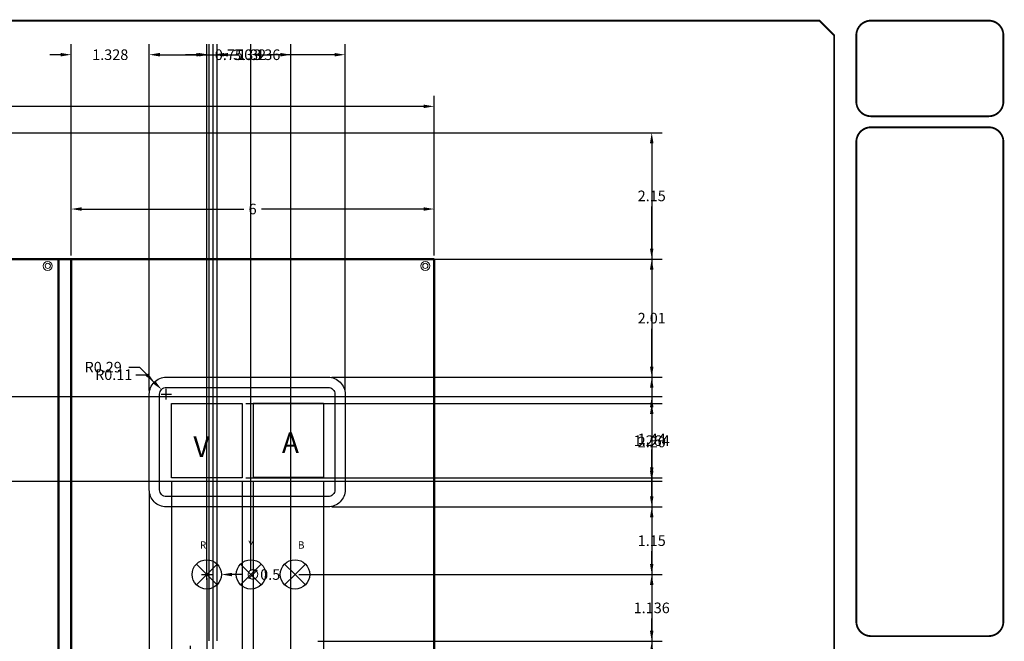
# Model space of a CAD drawing. Units: inches. Extents: x 0 to 33.5, y 0 to 22.4.
# Tile 6 of 6: x 16.8 to 33.5, y 11.9 to 22.4. Entities that reach past the tile are written whole.
import ezdxf
from ezdxf.enums import TextEntityAlignment as Align

# ---------------------------------------------------------------- set-up
doc = ezdxf.new("R2010")
doc.units = ezdxf.units.IN
doc.header["$MEASUREMENT"] = 0
for name, color, linetype, lineweight in [('E-ANNO-DIMS', 2, 'Continuous', 18), ('E-ANNO-TEXT', 7, 'Continuous', 18), ('E-ANNO-TTLB', 7, 'Continuous', 35), ('E-PANL-DEVC', 4, 'Continuous', 25), ('E-PANL-HDWR', 8, 'Continuous', 18), ('E-PANL-OUTL', 7, 'Continuous', 50)]:
    doc.layers.add(name, color=color, linetype=linetype, lineweight=lineweight)
doc.layers.add('TITLE', color=7, linetype='Continuous')
doc.styles.add('ITALIC', font='ITALIC')
doc.styles.add('SIMPLEX', font='SIMPLEX')
doc.dimstyles.get("Standard").update_dxf_attribs({"dimtxt": 0.18, "dimasz": 0.18, "dimexe": 0.18, "dimexo": 0.0625, "dimgap": 0.09, "dimtad": 0, "dimtih": 1, "dimtoh": 1, "dimdec": 0, "dimzin": 0, "dimdsep": 46, "dimtxsty": 'Standard', "dimcen": 0.09, "dimadec": 0, "dimazin": 0, "dimtfac": 1, "dimtdec": 0, "dimtofl": 0, "dimtmove": 0, "dimatfit": 3, "dimfxl": 1, "dimtolj": 1, "dimtzin": 0, "dimarcsym": 0})

# ---------------------------------------------------------------- blocks, each defined once
blk = doc.blocks.new('NO_NUM_acade_title')
at = {"layer": 'TITLE'}
blk.add_line((30.594, 22.177), (30.594, 20.781), dxfattribs=at)
at = {"layer": 'TITLE', "const_width": 0.0312}
blk.add_lwpolyline([(30.594, 0.281), (30.594, 22.177), (30.344, 22.427), (0.281, 22.427), (0.031, 22.177), (0.031, 0.281), (0.281, 0.031), (30.344, 0.031)], close=True, dxfattribs=at)
for points in [[(31.219, 22.427, 0.414214), (30.969, 22.177, 0.414214)], [(33.469, 22.177, 0.414214), (33.219, 22.427, 0.414214)], [(30.969, 21.052, 0.414214), (31.219, 20.802, 0.414214)], [(33.219, 20.802, 0.414214), (33.469, 21.052, 0.414214)], [(31.219, 20.615, 0.414214), (30.969, 20.365, 0.414214)], [(33.469, 20.365, 0.414214), (33.219, 20.615, 0.414214)], [(30.969, 12.219, 0.414214), (31.219, 11.969, 0.414214)], [(33.219, 11.969, 0.414214), (33.469, 12.219, 0.414214)]]:
    blk.add_lwpolyline(points, format="xyb", dxfattribs=at)
for points in [[(33.219, 22.427), (31.219, 22.427)], [(30.969, 22.177), (30.969, 21.052)], [(33.469, 22.177), (33.469, 21.052)], [(33.219, 20.802), (31.219, 20.802)], [(33.219, 20.615), (31.219, 20.615)], [(30.969, 20.365), (30.969, 12.219)], [(33.469, 20.365), (33.469, 12.219)], [(31.219, 11.969), (33.219, 11.969)]]:
    blk.add_lwpolyline(points, dxfattribs=at)
at = {"layer": 'TITLE', "style": 'ITALIC'}
for tag, height, p in [('TITLE#1', 0.125, (32.156, 3.406)), ('TITLE#2', 0.125, (32.156, 3.204)), ('TITLE#3', 0.125, (32.156, 3.001)), ('TITLE#4', 0.125, (32.156, 2.799)), ('DWG#', 0.2, (32.156, 0.826))]:
    blk.add_attdef(tag, text='', height=height, dxfattribs=at).set_placement(p, align=Align.CENTER)
at = {"layer": 'TITLE', "style": 'SIMPLEX'}
blk.add_attdef('CAD#', (30.826, 1.958), '', height=0.0938, rotation=90, dxfattribs=at)
at = {"layer": 'TITLE'}
for tag, p, height, style in [('JOB#', (31.464, 1.644), 0.0938, 'SIMPLEX'), ('SCALE', (31.353, 1.344), 0.0938, 'SIMPLEX'), ('DATE', (32.408, 1.344), 0.0938, 'SIMPLEX'), ('SHTS', (32.532, 0.25), 0.2, 'ITALIC')]:
    blk.add_attdef(tag, p, '', height=height, dxfattribs=dict(at, style=style))
at = {"layer": 'TITLE', "style": 'ITALIC'}
blk.add_attdef('SH#', text='', height=0.2, dxfattribs=at).set_placement((31.881, 0.25), align=Align.RIGHT)
at = {"layer": 'TITLE', "flags": 9}
blk.add_attdef('WD_TB', (31.219, 0.031), '', height=0.125, dxfattribs=at)
blk = doc.blocks.new('*D18')
at = {"layer": 'Defpoints', "color": 0, "transparency": 16777216}
for p in [(23.794, 20.97), (4.625, 18.375), (23.794, 18.375)]:
    blk.add_point(p, dxfattribs=at)
at = {"layer": 'E-ANNO-DIMS', "color": 0, "lineweight": -2, "transparency": 16777216}
for p, q in [((4.625, 18.438), (4.625, 21.15)), ((23.794, 18.438), (23.794, 21.15)), ((4.805, 20.97), (13.999, 20.97)), ((23.614, 20.97), (14.419, 20.97))]:
    blk.add_line(p, q, dxfattribs=at)
at = {"layer": 'E-ANNO-DIMS', "color": 0, "transparency": 16777216}
for points in [[(4.805, 21), (4.805, 20.94), (4.625, 20.97)], [(23.614, 21), (23.614, 20.94), (23.794, 20.97)]]:
    blk.add_solid(points, dxfattribs=at)
at = {"layer": 'E-ANNO-DIMS', "color": 0, "transparency": 16777216, "insert": (14.209, 20.97), "char_height": 0.18, "attachment_point": 5}
blk.add_mtext('\\A1;19', dxfattribs=at)
blk = doc.blocks.new('*D20')
at = {"layer": 'Defpoints', "color": 0, "transparency": 16777216}
for p in [(23.794, 19.226), (17.625, 18.375), (23.794, 18.375)]:
    blk.add_point(p, dxfattribs=at)
at = {"layer": 'E-ANNO-DIMS', "color": 0, "lineweight": -2, "transparency": 16777216}
for p, q in [((17.625, 18.438), (17.625, 19.406)), ((23.794, 18.438), (23.794, 19.406)), ((17.805, 19.226), (20.559, 19.226)), ((23.614, 19.226), (20.859, 19.226))]:
    blk.add_line(p, q, dxfattribs=at)
at = {"layer": 'E-ANNO-DIMS', "color": 0, "transparency": 16777216}
for points in [[(17.805, 19.256), (17.805, 19.196), (17.625, 19.226)], [(23.614, 19.256), (23.614, 19.196), (23.794, 19.226)]]:
    blk.add_solid(points, dxfattribs=at)
at = {"layer": 'E-ANNO-DIMS', "color": 0, "transparency": 16777216, "insert": (20.709, 19.226), "char_height": 0.18, "attachment_point": 5}
blk.add_mtext('\\A1;6', dxfattribs=at)
blk = doc.blocks.new('LAMP-IND')
for q in [(0.073, 0.427), (0.426, 0.427), (0.073, 0.073), (0.426, 0.073)]:
    blk.add_line((0.25, 0.25), q)
blk.add_circle((0.25, 0.25), 0.25)
blk = doc.blocks.new('SCREW-PANEL')
for radius in [0.0768, 0.0442]:
    blk.add_circle((0.077, 0.077), radius)
blk = doc.blocks.new('*D29')
at = {"layer": 'Defpoints', "color": 0, "transparency": 16777216}
for p in [(14.887, 20.523), (27.492, 20.523), (15.246, 18.375)]:
    blk.add_point(p, dxfattribs=at)
at = {"layer": 'E-ANNO-DIMS', "color": 0, "lineweight": -2, "transparency": 16777216}
for p, q in [((14.95, 20.523), (27.672, 20.523)), ((27.492, 20.343), (27.492, 19.629)), ((27.492, 18.555), (27.492, 19.269)), ((15.308, 18.375), (27.672, 18.375))]:
    blk.add_line(p, q, dxfattribs=at)
at = {"layer": 'E-ANNO-DIMS', "color": 0, "transparency": 16777216}
for points in [[(27.462, 20.343), (27.522, 20.343), (27.492, 20.523)], [(27.462, 18.555), (27.522, 18.555), (27.492, 18.375)]]:
    blk.add_solid(points, dxfattribs=at)
at = {"layer": 'E-ANNO-DIMS', "color": 0, "transparency": 16777216, "insert": (27.492, 19.449), "char_height": 0.18, "attachment_point": 5}
blk.add_mtext('\\A1;2.15', dxfattribs=at)
blk = doc.blocks.new('*D31')
at = {"layer": 'Defpoints', "color": 0, "transparency": 16777216}
for p in [(14.887335, 20.522539), (27.49197, 20.522539), (23.941819, 1.679641)]:
    blk.add_point(p, dxfattribs=at)
at = {"layer": 'E-ANNO-DIMS', "color": 0, "lineweight": -2, "transparency": 16777216}
for p, q in [((14.949835, 20.522539), (27.67197, 20.522539)), ((27.49197, 20.342539), (27.49197, 11.28109)), ((27.49197, 1.859641), (27.49197, 10.92109)), ((24.004319, 1.679641), (27.67197, 1.679641))]:
    blk.add_line(p, q, dxfattribs=at)
at = {"layer": 'E-ANNO-DIMS', "color": 0, "transparency": 16777216}
for points in [[(27.46197, 20.342539), (27.52197, 20.342539), (27.49197, 20.522539)], [(27.46197, 1.859641), (27.52197, 1.859641), (27.49197, 1.679641)]]:
    blk.add_solid(points, dxfattribs=at)
at = {"layer": 'E-ANNO-DIMS', "color": 0, "transparency": 16777216, "insert": (27.49197, 11.10109), "char_height": 0.18, "attachment_point": 5}
blk.add_mtext('\\A1;18.843', dxfattribs=at)
blk = doc.blocks.new('*D56')
at = {"layer": 'Defpoints', "color": 0, "transparency": 16777216}
for p in [(15.436773, 16.038508), (15.436773, 14.601008), (27.49197, 14.601008)]:
    blk.add_point(p, dxfattribs=at)
at = {"layer": 'E-ANNO-DIMS', "color": 0, "lineweight": -2, "transparency": 16777216}
for p, q in [((15.499273, 16.038508), (27.67197, 16.038508)), ((27.49197, 15.858508), (27.49197, 15.499758)), ((27.49197, 14.781008), (27.49197, 15.139758)), ((15.499273, 14.601008), (27.67197, 14.601008))]:
    blk.add_line(p, q, dxfattribs=at)
at = {"layer": 'E-ANNO-DIMS', "color": 0, "transparency": 16777216}
for points in [[(27.46197, 15.858508), (27.52197, 15.858508), (27.49197, 16.038508)], [(27.46197, 14.781008), (27.52197, 14.781008), (27.49197, 14.601008)]]:
    blk.add_solid(points, dxfattribs=at)
at = {"layer": 'E-ANNO-DIMS', "color": 0, "transparency": 16777216, "insert": (27.49197, 15.319758), "char_height": 0.18, "attachment_point": 5}
blk.add_mtext('\\A1;1.44', dxfattribs=at)
blk = doc.blocks.new('*D67')
at = {"layer": 'Defpoints', "color": 0, "transparency": 16777216}
for p in [(22.281399, 21.847539), (18.952991, 16.079443), (22.281399, 16.079443)]:
    blk.add_point(p, dxfattribs=at)
at = {"layer": 'E-ANNO-DIMS', "color": 0, "lineweight": -2, "transparency": 16777216}
for p, q in [((18.952991, 16.141943), (18.952991, 22.027539)), ((22.281399, 16.141943), (22.281399, 22.027539)), ((19.132991, 21.847539), (20.257195, 21.847539)), ((22.101399, 21.847539), (20.977195, 21.847539))]:
    blk.add_line(p, q, dxfattribs=at)
at = {"layer": 'E-ANNO-DIMS', "color": 0, "transparency": 16777216}
for points in [[(19.132991, 21.877539), (19.132991, 21.817539), (18.952991, 21.847539)], [(22.101399, 21.877539), (22.101399, 21.817539), (22.281399, 21.847539)]]:
    blk.add_solid(points, dxfattribs=at)
at = {"layer": 'E-ANNO-DIMS', "color": 0, "transparency": 16777216, "insert": (20.617195, 21.847539), "char_height": 0.18, "attachment_point": 5}
blk.add_mtext('\\A1;3.33', dxfattribs=at)
blk = doc.blocks.new('*D68')
at = {"layer": 'Defpoints', "color": 0, "transparency": 16777216}
for p in [(19.330943, 14.658017), (18.952991, 14.454443), (19.330943, 0.354641)]:
    blk.add_point(p, dxfattribs=at)
at = {"layer": 'E-ANNO-DIMS', "color": 0, "lineweight": -2, "transparency": 16777216}
for p, q in [((19.330943, 14.595517), (19.330943, 0.174641)), ((18.952991, 14.391943), (18.952991, 0.174641)), ((18.772991, 0.354641), (18.592991, 0.354641)), ((19.510943, 0.354641), (19.690943, 0.354641))]:
    blk.add_line(p, q, dxfattribs=at)
at = {"layer": 'E-ANNO-DIMS', "color": 0, "transparency": 16777216}
for points in [[(18.772991, 0.384641), (18.772991, 0.324641), (18.952991, 0.354641)], [(19.510943, 0.384641), (19.510943, 0.324641), (19.330943, 0.354641)]]:
    blk.add_solid(points, dxfattribs=at)
at = {"layer": 'E-ANNO-DIMS', "color": 0, "transparency": 16777216, "insert": (20.125943, 0.354641), "char_height": 0.18, "attachment_point": 5}
blk.add_mtext('\\A1;0.378', dxfattribs=at)
blk = doc.blocks.new('*D69')
at = {"layer": 'Defpoints', "color": 0, "transparency": 16777216}
for p in [(19.330943, 14.658017), (20.529167, 14.658017), (20.529167, 0.354641)]:
    blk.add_point(p, dxfattribs=at)
at = {"layer": 'E-ANNO-DIMS', "color": 0, "lineweight": -2, "transparency": 16777216}
for p, q in [((19.330943, 14.595517), (19.330943, 0.174641)), ((20.529167, 14.595517), (20.529167, 0.174641)), ((19.510943, 0.354641), (19.615055, 0.354641)), ((20.349167, 0.354641), (20.245055, 0.354641))]:
    blk.add_line(p, q, dxfattribs=at)
at = {"layer": 'E-ANNO-DIMS', "color": 0, "transparency": 16777216}
for points in [[(19.510943, 0.384641), (19.510943, 0.324641), (19.330943, 0.354641)], [(20.349167, 0.384641), (20.349167, 0.324641), (20.529167, 0.354641)]]:
    blk.add_solid(points, dxfattribs=at)
at = {"layer": 'E-ANNO-DIMS', "color": 0, "transparency": 16777216, "insert": (19.930055, 0.354641), "char_height": 0.18, "attachment_point": 5}
blk.add_mtext('\\A1;1.20', dxfattribs=at)
blk = doc.blocks.new('*D70')
at = {"layer": 'Defpoints', "color": 0, "transparency": 16777216}
for p in [(20.529167, 14.658017), (20.716317, 14.66483), (20.716317, 0.354641)]:
    blk.add_point(p, dxfattribs=at)
at = {"layer": 'E-ANNO-DIMS', "color": 0, "lineweight": -2, "transparency": 16777216}
for p, q in [((20.529167, 14.595517), (20.529167, 0.174641)), ((20.716317, 14.60233), (20.716317, 0.174641)), ((20.349167, 0.354641), (20.169167, 0.354641)), ((20.896317, 0.354641), (21.076317, 0.354641))]:
    blk.add_line(p, q, dxfattribs=at)
at = {"layer": 'E-ANNO-DIMS', "color": 0, "transparency": 16777216}
for points in [[(20.349167, 0.384641), (20.349167, 0.324641), (20.529167, 0.354641)], [(20.896317, 0.384641), (20.896317, 0.324641), (20.716317, 0.354641)]]:
    blk.add_solid(points, dxfattribs=at)
at = {"layer": 'E-ANNO-DIMS', "color": 0, "transparency": 16777216, "insert": (21.391317, 0.354641), "char_height": 0.18, "attachment_point": 5}
blk.add_mtext('\\A1;0.19', dxfattribs=at)
blk = doc.blocks.new('*D71')
at = {"layer": 'Defpoints', "color": 0, "transparency": 16777216}
for p in [(20.716, 14.665), (21.915, 14.665), (21.915, 0.355)]:
    blk.add_point(p, dxfattribs=at)
at = {"layer": 'E-ANNO-DIMS', "color": 0, "lineweight": -2, "transparency": 16777216}
for p, q in [((20.716, 14.602), (20.716, 0.175)), ((21.915, 14.602), (21.915, 0.175)), ((20.896, 0.355), (21, 0.355)), ((21.735, 0.355), (21.63, 0.355))]:
    blk.add_line(p, q, dxfattribs=at)
at = {"layer": 'E-ANNO-DIMS', "color": 0, "transparency": 16777216}
for points in [[(20.896, 0.385), (20.896, 0.325), (20.716, 0.355)], [(21.735, 0.385), (21.735, 0.325), (21.915, 0.355)]]:
    blk.add_solid(points, dxfattribs=at)
at = {"layer": 'E-ANNO-DIMS', "color": 0, "transparency": 16777216, "insert": (21.315, 0.355), "char_height": 0.18, "attachment_point": 5}
blk.add_mtext('\\A1;1.20', dxfattribs=at)
blk = doc.blocks.new('*D72')
at = {"layer": 'Defpoints', "color": 0, "transparency": 16777216}
for p in [(20.529, 15.922), (20.529, 14.658), (27.492, 14.658)]:
    blk.add_point(p, dxfattribs=at)
at = {"layer": 'E-ANNO-DIMS', "color": 0, "lineweight": -2, "transparency": 16777216}
for p, q in [((20.592, 15.922), (27.672, 15.922)), ((27.492, 15.742), (27.492, 15.47)), ((27.492, 14.838), (27.492, 15.11)), ((20.592, 14.658), (27.672, 14.658))]:
    blk.add_line(p, q, dxfattribs=at)
at = {"layer": 'E-ANNO-DIMS', "color": 0, "transparency": 16777216}
for points in [[(27.462, 15.742), (27.522, 15.742), (27.492, 15.922)], [(27.462, 14.838), (27.522, 14.838), (27.492, 14.658)]]:
    blk.add_solid(points, dxfattribs=at)
at = {"layer": 'E-ANNO-DIMS', "color": 0, "transparency": 16777216, "insert": (27.492, 15.29), "char_height": 0.18, "attachment_point": 5}
blk.add_mtext('\\A1;1.264', dxfattribs=at)
blk = doc.blocks.new('*D73')
at = {"layer": 'Defpoints', "color": 0, "transparency": 16777216}
for p in [(18.953, 21.848), (17.625, 18.375), (18.953, 16.079)]:
    blk.add_point(p, dxfattribs=at)
at = {"layer": 'E-ANNO-DIMS', "color": 0, "lineweight": -2, "transparency": 16777216}
for p, q in [((17.625, 18.438), (17.625, 22.028)), ((18.953, 16.142), (18.953, 22.028)), ((17.445, 21.848), (17.265, 21.848)), ((19.133, 21.848), (19.313, 21.848))]:
    blk.add_line(p, q, dxfattribs=at)
at = {"layer": 'E-ANNO-DIMS', "color": 0, "transparency": 16777216}
for points in [[(17.445, 21.878), (17.445, 21.818), (17.625, 21.848)], [(19.133, 21.878), (19.133, 21.818), (18.953, 21.848)]]:
    blk.add_solid(points, dxfattribs=at)
at = {"layer": 'E-ANNO-DIMS', "color": 0, "transparency": 16777216, "insert": (18.289, 21.848), "char_height": 0.18, "attachment_point": 5}
blk.add_mtext('\\A1;1.328', dxfattribs=at)
blk = doc.blocks.new('*D74')
at = {"layer": 'Defpoints', "color": 0, "transparency": 16777216}
for p in [(17.625, 18.375), (19.93, 13.017), (19.93, 0.355)]:
    blk.add_point(p, dxfattribs=at)
at = {"layer": 'E-ANNO-DIMS', "color": 0, "lineweight": -2, "transparency": 16777216}
for p, q in [((17.625, 18.312), (17.625, 0.175)), ((19.93, 12.954), (19.93, 0.175)), ((17.805, 0.355), (18.432, 0.355)), ((19.75, 0.355), (19.122, 0.355))]:
    blk.add_line(p, q, dxfattribs=at)
at = {"layer": 'E-ANNO-DIMS', "color": 0, "transparency": 16777216}
for points in [[(17.805, 0.385), (17.805, 0.325), (17.625, 0.355)], [(19.75, 0.385), (19.75, 0.325), (19.93, 0.355)]]:
    blk.add_solid(points, dxfattribs=at)
at = {"layer": 'E-ANNO-DIMS', "color": 0, "transparency": 16777216, "insert": (18.777, 0.355), "char_height": 0.18, "attachment_point": 5}
blk.add_mtext('\\A1;2.30', dxfattribs=at)
blk = doc.blocks.new('*D75')
at = {"layer": 'Defpoints', "color": 0, "transparency": 16777216}
for p in [(20.679695, 21.847539), (19.929695, 13.016943), (20.679695, 13.016943)]:
    blk.add_point(p, dxfattribs=at)
at = {"layer": 'E-ANNO-DIMS', "color": 0, "lineweight": -2, "transparency": 16777216}
for p, q in [((19.929695, 13.079443), (19.929695, 22.027539)), ((20.679695, 13.079443), (20.679695, 22.027539)), ((19.749695, 21.847539), (19.569695, 21.847539)), ((20.859695, 21.847539), (21.039695, 21.847539))]:
    blk.add_line(p, q, dxfattribs=at)
at = {"layer": 'E-ANNO-DIMS', "color": 0, "transparency": 16777216}
for points in [[(19.749695, 21.877539), (19.749695, 21.817539), (19.929695, 21.847539)], [(20.859695, 21.877539), (20.859695, 21.817539), (20.679695, 21.847539)]]:
    blk.add_solid(points, dxfattribs=at)
at = {"layer": 'E-ANNO-DIMS', "color": 0, "transparency": 16777216, "insert": (20.304695, 21.847539), "char_height": 0.18, "attachment_point": 5}
blk.add_mtext('\\A1;0.75', dxfattribs=at)
blk = doc.blocks.new('*D76')
at = {"layer": 'Defpoints', "color": 0, "transparency": 16777216}
for p in [(23.793662, 18.375), (21.992195, 16.368648), (27.49197, 16.368648)]:
    blk.add_point(p, dxfattribs=at)
at = {"layer": 'E-ANNO-DIMS', "color": 0, "lineweight": -2, "transparency": 16777216}
for p, q in [((23.856162, 18.375), (27.67197, 18.375)), ((27.49197, 18.195), (27.49197, 17.551824)), ((27.49197, 16.548648), (27.49197, 17.191824)), ((22.054695, 16.368648), (27.67197, 16.368648))]:
    blk.add_line(p, q, dxfattribs=at)
at = {"layer": 'E-ANNO-DIMS', "color": 0, "transparency": 16777216}
for points in [[(27.46197, 18.195), (27.52197, 18.195), (27.49197, 18.375)], [(27.46197, 16.548648), (27.52197, 16.548648), (27.49197, 16.368648)]]:
    blk.add_solid(points, dxfattribs=at)
at = {"layer": 'E-ANNO-DIMS', "color": 0, "transparency": 16777216, "insert": (27.49197, 17.371824), "char_height": 0.18, "attachment_point": 5}
blk.add_mtext('\\A1;2.01', dxfattribs=at)
blk = doc.blocks.new('*D77')
at = {"layer": 'Defpoints', "color": 0, "transparency": 16777216}
for p in [(21.992, 16.369), (21.992, 14.165), (27.492, 14.165)]:
    blk.add_point(p, dxfattribs=at)
at = {"layer": 'E-ANNO-DIMS', "color": 0, "lineweight": -2, "transparency": 16777216}
for p, q in [((22.055, 16.369), (27.672, 16.369)), ((27.492, 16.189), (27.492, 15.447)), ((27.492, 14.345), (27.492, 15.087)), ((22.055, 14.165), (27.672, 14.165))]:
    blk.add_line(p, q, dxfattribs=at)
at = {"layer": 'E-ANNO-DIMS', "color": 0, "transparency": 16777216}
for points in [[(27.462, 16.189), (27.522, 16.189), (27.492, 16.369)], [(27.462, 14.345), (27.522, 14.345), (27.492, 14.165)]]:
    blk.add_solid(points, dxfattribs=at)
at = {"layer": 'E-ANNO-DIMS', "color": 0, "transparency": 16777216, "insert": (27.492, 15.267), "char_height": 0.18, "attachment_point": 5}
blk.add_mtext('\\A1;2.20', dxfattribs=at)
blk = doc.blocks.new('*D78')
at = {"layer": 'Defpoints', "color": 0, "transparency": 16777216}
for p in [(21.992195, 14.165239), (21.429695, 13.016943), (27.49197, 13.016943)]:
    blk.add_point(p, dxfattribs=at)
at = {"layer": 'E-ANNO-DIMS', "color": 0, "lineweight": -2, "transparency": 16777216}
for p, q in [((22.054695, 14.165239), (27.67197, 14.165239)), ((27.49197, 13.985239), (27.49197, 13.771091)), ((27.49197, 13.196943), (27.49197, 13.411091)), ((21.492195, 13.016943), (27.67197, 13.016943))]:
    blk.add_line(p, q, dxfattribs=at)
at = {"layer": 'E-ANNO-DIMS', "color": 0, "transparency": 16777216}
for points in [[(27.46197, 13.985239), (27.52197, 13.985239), (27.49197, 14.165239)], [(27.46197, 13.196943), (27.52197, 13.196943), (27.49197, 13.016943)]]:
    blk.add_solid(points, dxfattribs=at)
at = {"layer": 'E-ANNO-DIMS', "color": 0, "transparency": 16777216, "insert": (27.49197, 13.591091), "char_height": 0.18, "attachment_point": 5}
blk.add_mtext('\\A1;1.15', dxfattribs=at)
blk = doc.blocks.new('*D79')
at = {"layer": 'Defpoints', "color": 0, "transparency": 16777216}
for p in [(21.429695, 13.016943), (21.753278, 11.880921), (27.49197, 11.880921)]:
    blk.add_point(p, dxfattribs=at)
at = {"layer": 'E-ANNO-DIMS', "color": 0, "lineweight": -2, "transparency": 16777216}
for p, q in [((21.492195, 13.016943), (27.67197, 13.016943)), ((27.49197, 12.836943), (27.49197, 12.628932)), ((27.49197, 12.060921), (27.49197, 12.268932)), ((21.815778, 11.880921), (27.67197, 11.880921))]:
    blk.add_line(p, q, dxfattribs=at)
at = {"layer": 'E-ANNO-DIMS', "color": 0, "transparency": 16777216}
for points in [[(27.46197, 12.836943), (27.52197, 12.836943), (27.49197, 13.016943)], [(27.46197, 12.060921), (27.52197, 12.060921), (27.49197, 11.880921)]]:
    blk.add_solid(points, dxfattribs=at)
at = {"layer": 'E-ANNO-DIMS', "color": 0, "transparency": 16777216, "insert": (27.49197, 12.448932), "char_height": 0.18, "attachment_point": 5}
blk.add_mtext('\\A1;1.136', dxfattribs=at)
blk = doc.blocks.new('*D80')
at = {"layer": 'Defpoints', "color": 0, "transparency": 16777216}
for p in [(21.753278, 11.880921), (21.753278, 11.05915), (27.49197, 11.05915)]:
    blk.add_point(p, dxfattribs=at)
at = {"layer": 'E-ANNO-DIMS', "color": 0, "lineweight": -2, "transparency": 16777216}
for p, q in [((21.815778, 11.880921), (27.67197, 11.880921)), ((27.49197, 11.700921), (27.49197, 11.23915)), ((21.815778, 11.05915), (27.67197, 11.05915)), ((27.49197, 11.05915), (27.49197, 10.87915)), ((27.49197, 10.87915), (27.31197, 10.87915))]:
    blk.add_line(p, q, dxfattribs=at)
at = {"layer": 'E-ANNO-DIMS', "color": 0, "transparency": 16777216}
for points in [[(27.46197, 11.700921), (27.52197, 11.700921), (27.49197, 11.880921)], [(27.46197, 11.23915), (27.52197, 11.23915), (27.49197, 11.05915)]]:
    blk.add_solid(points, dxfattribs=at)
at = {"layer": 'E-ANNO-DIMS', "color": 0, "transparency": 16777216, "insert": (26.96697, 10.87915), "char_height": 0.18, "attachment_point": 5}
blk.add_mtext('\\A1;0.82', dxfattribs=at)
blk = doc.blocks.new('*D82')
at = {"layer": 'Defpoints', "color": 0, "transparency": 16777216}
for p in [(17.625, 18.375), (19.645494, 11.8638), (19.645494, 0.354641)]:
    blk.add_point(p, dxfattribs=at)
at = {"layer": 'E-ANNO-DIMS', "color": 0, "lineweight": -2, "transparency": 16777216}
for p, q in [((17.625, 18.3125), (17.625, 0.174641)), ((19.645494, 11.8013), (19.645494, 0.174641)), ((17.805, 0.354641), (18.290247, 0.354641)), ((19.465494, 0.354641), (18.980247, 0.354641))]:
    blk.add_line(p, q, dxfattribs=at)
at = {"layer": 'E-ANNO-DIMS', "color": 0, "transparency": 16777216}
for points in [[(17.805, 0.384641), (17.805, 0.324641), (17.625, 0.354641)], [(19.465494, 0.384641), (19.465494, 0.324641), (19.645494, 0.354641)]]:
    blk.add_solid(points, dxfattribs=at)
at = {"layer": 'E-ANNO-DIMS', "color": 0, "transparency": 16777216, "insert": (18.635247, 0.354641), "char_height": 0.18, "attachment_point": 5}
blk.add_mtext('\\A1;2.02', dxfattribs=at)
blk = doc.blocks.new('*D83')
at = {"layer": 'Defpoints', "color": 0, "transparency": 16777216}
for p in [(17.625, 18.375), (20.989, 8.496), (20.989, 0.355)]:
    blk.add_point(p, dxfattribs=at)
at = {"layer": 'E-ANNO-DIMS', "color": 0, "lineweight": -2, "transparency": 16777216}
for p, q in [((17.625, 18.312), (17.625, 0.175)), ((20.989, 8.433), (20.989, 0.175)), ((17.805, 0.355), (18.947, 0.355)), ((20.809, 0.355), (19.667, 0.355))]:
    blk.add_line(p, q, dxfattribs=at)
at = {"layer": 'E-ANNO-DIMS', "color": 0, "transparency": 16777216}
for points in [[(17.805, 0.385), (17.805, 0.325), (17.625, 0.355)], [(20.809, 0.385), (20.809, 0.325), (20.989, 0.355)]]:
    blk.add_solid(points, dxfattribs=at)
at = {"layer": 'E-ANNO-DIMS', "color": 0, "transparency": 16777216, "insert": (19.307, 0.355), "char_height": 0.18, "attachment_point": 5}
blk.add_mtext('\\A1;3.36', dxfattribs=at)
blk = doc.blocks.new('*D84')
at = {"layer": 'Defpoints', "color": 0, "transparency": 16777216}
for p in [(21.35914, 21.847539), (20.039632, 11.452915), (21.35914, 11.470035)]:
    blk.add_point(p, dxfattribs=at)
at = {"layer": 'E-ANNO-DIMS', "color": 0, "lineweight": -2, "transparency": 16777216}
for p, q in [((20.039632, 11.515415), (20.039632, 22.027539)), ((21.35914, 11.532535), (21.35914, 22.027539)), ((20.219632, 21.847539), (20.369386, 21.847539)), ((21.17914, 21.847539), (21.029386, 21.847539))]:
    blk.add_line(p, q, dxfattribs=at)
at = {"layer": 'E-ANNO-DIMS', "color": 0, "transparency": 16777216}
for points in [[(20.219632, 21.877539), (20.219632, 21.817539), (20.039632, 21.847539)], [(21.17914, 21.877539), (21.17914, 21.817539), (21.35914, 21.847539)]]:
    blk.add_solid(points, dxfattribs=at)
at = {"layer": 'E-ANNO-DIMS', "color": 0, "transparency": 16777216, "insert": (20.699386, 21.847539), "char_height": 0.18, "attachment_point": 5}
blk.add_mtext('\\A1;1.32', dxfattribs=at)
blk = doc.blocks.new('*D85')
at = {"layer": 'Defpoints', "color": 0, "transparency": 16777216}
for p in [(20.108027, 21.847539), (19.972101, 11.828212), (20.108027, 11.828212)]:
    blk.add_point(p, dxfattribs=at)
at = {"layer": 'E-ANNO-DIMS', "color": 0, "lineweight": -2, "transparency": 16777216}
for p, q in [((19.972101, 11.890712), (19.972101, 22.027539)), ((20.108027, 11.890712), (20.108027, 22.027539)), ((19.792101, 21.847539), (19.612101, 21.847539)), ((20.288027, 21.847539), (20.468027, 21.847539))]:
    blk.add_line(p, q, dxfattribs=at)
at = {"layer": 'E-ANNO-DIMS', "color": 0, "transparency": 16777216}
for points in [[(19.792101, 21.877539), (19.792101, 21.817539), (19.972101, 21.847539)], [(20.288027, 21.877539), (20.288027, 21.817539), (20.108027, 21.847539)]]:
    blk.add_solid(points, dxfattribs=at)
at = {"layer": 'E-ANNO-DIMS', "color": 0, "transparency": 16777216, "insert": (20.873027, 21.847539), "char_height": 0.18, "attachment_point": 5}
blk.add_mtext('\\A1;0.136', dxfattribs=at)
blk = doc.blocks.new('*D95')
at = {"layer": 'Defpoints', "color": 0, "transparency": 16777216}
for p in [(19.038, 16.284), (19.242, 16.079)]:
    blk.add_point(p, dxfattribs=at)
at = {"layer": 'E-ANNO-DIMS', "color": 0, "lineweight": -2, "transparency": 16777216}
for p, q in [((18.604, 16.539), (18.784, 16.539)), ((18.784, 16.539), (18.911, 16.412)), ((19.152, 16.079), (19.332, 16.079)), ((19.242, 15.989), (19.242, 16.169))]:
    blk.add_line(p, q, dxfattribs=at)
at = {"layer": 'E-ANNO-DIMS', "color": 0, "transparency": 16777216}
blk.add_solid([(18.932, 16.433), (18.889, 16.39), (19.038, 16.284)], dxfattribs=at)
at = {"layer": 'E-ANNO-DIMS', "color": 0, "transparency": 16777216, "insert": (18.169, 16.539), "char_height": 0.18, "attachment_point": 5}
blk.add_mtext('\\A1;R0.29', dxfattribs=at)
blk = doc.blocks.new('*D96')
at = {"layer": 'Defpoints', "color": 0, "transparency": 16777216}
for p in [(19.161, 16.159), (19.242, 16.079)]:
    blk.add_point(p, dxfattribs=at)
at = {"layer": 'E-ANNO-DIMS', "color": 0, "lineweight": -2, "transparency": 16777216}
for p, q in [((18.723, 16.411), (18.903, 16.411)), ((18.903, 16.411), (19.032, 16.285)), ((19.152, 16.079), (19.332, 16.079)), ((19.242, 15.989), (19.242, 16.169))]:
    blk.add_line(p, q, dxfattribs=at)
at = {"layer": 'E-ANNO-DIMS', "color": 0, "transparency": 16777216}
blk.add_solid([(19.053, 16.307), (19.011, 16.264), (19.161, 16.159)], dxfattribs=at)
at = {"layer": 'E-ANNO-DIMS', "color": 0, "transparency": 16777216, "insert": (18.348, 16.411), "char_height": 0.18, "attachment_point": 5}
blk.add_mtext('\\A1;R0.11', dxfattribs=at)
blk = doc.blocks.new('*D97')
at = {"layer": 'Defpoints', "color": 0, "transparency": 16777216}
for p in [(19.68, 13.018), (20.18, 13.016)]:
    blk.add_point(p, dxfattribs=at)
at = {"layer": 'E-ANNO-DIMS', "color": 0, "lineweight": -2, "transparency": 16777216}
for p, q in [((19.93, 12.927), (19.93, 13.107)), ((19.84, 13.017), (20.02, 13.017)), ((20.54, 13.015), (20.36, 13.015))]:
    blk.add_line(p, q, dxfattribs=at)
at = {"layer": 'E-ANNO-DIMS', "color": 0, "transparency": 16777216}
blk.add_solid([(20.36, 13.045), (20.36, 12.985), (20.18, 13.016)], dxfattribs=at)
at = {"layer": 'E-ANNO-DIMS', "color": 0, "transparency": 16777216, "insert": (20.885, 13.015), "char_height": 0.18, "attachment_point": 5}
blk.add_mtext('\\A1;∅0.5', dxfattribs=at)

msp = doc.modelspace()

# ---------------------------------------------------------------- linework, layer by layer
at = {"layer": 'E-PANL-DEVC'}
for p, q in [((20.5292, 15.9221), (20.5292, 14.658)), ((20.7163, 15.929), (20.7163, 14.6648))]:
    msp.add_line(p, q, dxfattribs=at)
for points in [[(18.953, 16.0794, -0.4142136), (19.2422, 16.3686), (21.9922, 16.3686, -0.4142136), (22.2814, 16.0794), (22.2814, 14.4544, -0.4142136), (21.9922, 14.1652), (19.2422, 14.1652, -0.4142136), (18.953, 14.4544)], [(19.128, 16.0794, -0.4142136), (19.2422, 16.1936), (21.9922, 16.1936, -0.4142136), (22.1064, 16.0794), (22.1064, 14.4544, -0.4142136), (21.9922, 14.3403), (19.2422, 14.3403, -0.4142136), (19.128, 14.4544)]]:
    msp.add_lwpolyline(points, format="xyb", close=True, dxfattribs=at)
for points in [[(20.5292, 14.658), (19.3309, 14.658), (19.3309, 15.9221), (20.5292, 15.9221)], [(20.7163, 15.929), (21.9145, 15.929), (21.9145, 14.6648), (20.7163, 14.6648)]]:
    msp.add_lwpolyline(points, dxfattribs=at)
at = {"layer": 'E-PANL-OUTL'}
for p, q in [((4.6251, 18.375), (23.7937, 18.375)), ((17.4101, 3.5899), (17.4101, 18.375)), ((17.625, 3.5899), (17.625, 18.375)), ((23.7937, 3.375), (23.7937, 18.375))]:
    msp.add_line(p, q, dxfattribs=at)

# ---------------------------------------------------------------- block references
at = {"layer": 'E-ANNO-TTLB'}
msp.add_blockref('NO_NUM_acade_title', (0, 0), dxfattribs=at)
at = {"layer": 'E-PANL-DEVC'}
for p, rotation in [((20.1796, 12.7672), 89.99999999999883), ((20.9296, 12.7672), 90), ((21.6796, 12.7672), 89.99999999999945)]:
    msp.add_blockref('LAMP-IND', p, dxfattribs=dict(at, rotation=rotation))
at = {"layer": 'E-PANL-HDWR'}
for p in [(17.1499, 18.182), (23.5664, 18.182)]:
    msp.add_blockref('SCREW-PANEL', p, dxfattribs=at)

# ---------------------------------------------------------------- texts
at = {"layer": 'E-ANNO-TEXT'}
for s, p in [('A', (21.206, 15.0798)), ('V', (19.7009, 15.0149))]:
    msp.add_text(s, height=0.3511, dxfattribs=at).set_placement(p)
for s, p in [('R', (19.8672, 13.4544)), ('Y', (20.6812, 13.4662)), ('B', (21.5339, 13.4544))]:
    msp.add_text(s, height=0.125, dxfattribs=at).set_placement(p, align=Align.CENTER)

# ---------------------------------------------------------------- dimensions: what is measured, and where the dimension line sits
at = {"layer": 'E-ANNO-DIMS'}
for base, p1, p2, override, picture, middle in [((18.953, 21.8475), (17.625, 18.375), (18.953, 16.0794), {"dimdec": 3, "dimlfac": 1, "dimrnd": 0, "dimzin": 0, "dimdsep": 46, "dimlunit": 2}, '*D73', (18.289, 21.8475)), ((22.2814, 21.8475), (18.953, 16.0794), (22.2814, 16.0794), {"dimdec": 2, "dimlfac": 1, "dimrnd": 0, "dimzin": 0, "dimdsep": 46, "dimlunit": 2}, '*D67', (20.6172, 21.8475)), ((20.6797, 21.8475), (19.9297, 13.0169), (20.6797, 13.0169), {"dimdec": 2, "dimlfac": 1, "dimrnd": 0, "dimzin": 0, "dimdsep": 46, "dimlunit": 2}, '*D75', (20.3047, 21.8475)), ((20.108, 21.8475), (19.9721, 11.8282), (20.108, 11.8282), {"dimdec": 3, "dimlfac": 1, "dimrnd": 0, "dimzin": 0, "dimdsep": 46, "dimlunit": 2}, '*D85', (20.873, 21.8475)), ((21.3591, 21.8475), (20.0396, 11.4529), (21.3591, 11.47), {"dimdec": 2, "dimlfac": 1, "dimrnd": 0, "dimzin": 0, "dimdsep": 46, "dimlunit": 2}, '*D84', (20.6994, 21.8475)), ((23.7937, 20.9702), (4.6251, 18.375), (23.7937, 18.375), {"dimclrd": 0, "dimclre": 0, "dimclrt": 0}, '*D18', (14.2094, 20.9702)), ((23.7937, 19.2258), (17.625, 18.375), (23.7937, 18.375), {"dimclrd": 0, "dimclre": 0, "dimclrt": 0}, '*D20', (20.7093, 19.2258)), ((19.9297, 0.3546), (17.625, 18.375), (19.9297, 13.0169), {"dimdec": 2, "dimlfac": 1, "dimrnd": 0, "dimzin": 0, "dimdsep": 46, "dimlunit": 2}, '*D74', (18.7773, 0.3546)), ((19.6455, 0.3546), (17.625, 18.375), (19.6455, 11.8638), {"dimdec": 2, "dimlfac": 1, "dimrnd": 0, "dimzin": 0, "dimdsep": 46, "dimlunit": 2}, '*D82', (18.6352, 0.3546)), ((20.9894, 0.3546), (17.625, 18.375), (20.9894, 8.4958), {"dimdec": 2, "dimlfac": 1, "dimrnd": 0, "dimzin": 0, "dimdsep": 46, "dimlunit": 2}, '*D83', (19.3072, 0.3546)), ((19.3309, 0.3546), (18.953, 14.4544), (19.3309, 14.658), {"dimdec": 3, "dimlfac": 1, "dimrnd": 0, "dimzin": 0, "dimdsep": 46, "dimlunit": 2}, '*D68', (20.1259, 0.3546)), ((20.5292, 0.3546), (19.3309, 14.658), (20.5292, 14.658), {"dimdec": 2, "dimlfac": 1, "dimrnd": 0, "dimzin": 0, "dimdsep": 46, "dimlunit": 2}, '*D69', (19.9301, 0.3546)), ((20.7163, 0.3546), (20.5292, 14.658), (20.7163, 14.6648), {"dimdec": 2, "dimlfac": 1, "dimrnd": 0, "dimzin": 0, "dimdsep": 46, "dimlunit": 2}, '*D70', (21.3913, 0.3546)), ((21.9145, 0.3546), (20.7163, 14.6648), (21.9145, 14.6648), {"dimdec": 2, "dimlfac": 1, "dimrnd": 0, "dimzin": 0, "dimdsep": 46, "dimlunit": 2}, '*D71', (21.3154, 0.3546))]:
    dim = msp.add_linear_dim(base=base, p1=p1, p2=p2, dimstyle='Standard', override=override, dxfattribs=at)
    dim.commit()
    dim.dimension.update_dxf_attribs({"geometry": picture, "text_midpoint": middle})
for base, p1, p2, override, picture, middle in [((27.492, 20.5225), (15.2456, 18.375), (14.8873, 20.5225), {"dimdec": 2, "dimlfac": 1, "dimrnd": 0, "dimzin": 0, "dimdsep": 46, "dimlunit": 2}, '*D29', (27.492, 19.4488)), ((27.492, 20.5225), (23.9418, 1.6796), (14.8873, 20.5225), {"dimdec": 3, "dimlfac": 1, "dimrnd": 0, "dimzin": 0, "dimdsep": 46, "dimlunit": 2}, '*D31', (27.492, 11.1011)), ((27.492, 16.3686), (23.7937, 18.375), (21.9922, 16.3686), {"dimdec": 2, "dimlfac": 1, "dimrnd": 0, "dimzin": 0, "dimdsep": 46, "dimlunit": 2}, '*D76', (27.492, 17.3718)), ((27.492, 14.1652), (21.9922, 16.3686), (21.9922, 14.1652), {"dimdec": 2, "dimlfac": 1, "dimrnd": 0, "dimzin": 0, "dimdsep": 46, "dimlunit": 2}, '*D77', (27.492, 15.2669)), ((27.492, 14.601), (15.4368, 16.0385), (15.4368, 14.601), {"dimdec": 2, "dimlfac": 1, "dimrnd": 0, "dimzin": 0, "dimdsep": 46, "dimlunit": 2}, '*D56', (27.492, 15.3198)), ((27.492, 14.658), (20.5292, 15.9221), (20.5292, 14.658), {"dimdec": 3, "dimlfac": 1, "dimrnd": 0, "dimzin": 0, "dimdsep": 46, "dimlunit": 2}, '*D72', (27.492, 15.2901)), ((27.492, 13.0169), (21.9922, 14.1652), (21.4297, 13.0169), {"dimdec": 2, "dimlfac": 1, "dimrnd": 0, "dimzin": 0, "dimdsep": 46, "dimlunit": 2}, '*D78', (27.492, 13.5911)), ((27.492, 11.8809), (21.4297, 13.0169), (21.7533, 11.8809), {"dimdec": 3, "dimlfac": 1, "dimrnd": 0, "dimzin": 0, "dimdsep": 46, "dimlunit": 2}, '*D79', (27.492, 12.4489)), ((27.492, 11.0592), (21.7533, 11.8809), (21.7533, 11.0592), {"dimdec": 2, "dimlfac": 1, "dimrnd": 0, "dimzin": 0, "dimdsep": 46, "dimlunit": 2}, '*D80', (26.967, 10.8791))]:
    dim = msp.add_linear_dim(base=base, p1=p1, p2=p2, angle=90, dimstyle='Standard', override=override, dxfattribs=at)
    dim.commit()
    dim.dimension.update_dxf_attribs({"geometry": picture, "text_midpoint": middle})
for mpoint, picture, middle in [((19.0379, 16.2841), '*D95', (18.1685, 16.5389)), ((19.1606, 16.1593), '*D96', (18.3484, 16.4112))]:
    dim = msp.add_radius_dim(center=(19.2422, 16.0794), mpoint=mpoint, dimstyle='Standard', override={"dimdec": 2, "dimlfac": 1, "dimrnd": 0, "dimzin": 0, "dimdsep": 46, "dimlunit": 2}, dxfattribs=at)
    dim.commit()
    dim.dimension.update_dxf_attribs({"geometry": picture, "text_midpoint": middle})
dim = msp.add_diameter_dim_2p(p1=(19.6797, 13.0179), p2=(20.1797, 13.016), dimstyle='Standard', override={"dimdec": 1, "dimlfac": 1, "dimrnd": 0, "dimzin": 0, "dimdsep": 46, "dimlunit": 2}, dxfattribs=at)
dim.commit()
dim.dimension.update_dxf_attribs({"geometry": '*D97', "text_midpoint": (20.5397, 13.0146)})

doc.saveas('drawing.dxf')
